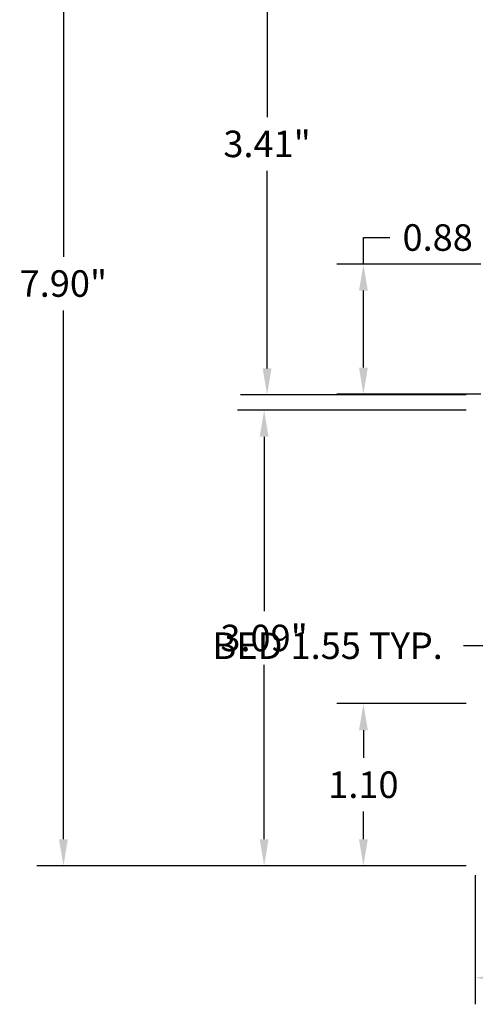
# Model space of a CAD drawing. Units: metres. Extents: x -1.9 to 13.1, y 0.9 to 14.8.
# Tile 1 of 7: x -1.9 to 1.2, y 1.8 to 8.4. Entities that reach past the tile are written whole.
import ezdxf

# ---------------------------------------------------------------- set-up
doc = ezdxf.new("R2010")
doc.units = ezdxf.units.M
doc.header["$MEASUREMENT"] = 0
doc.layers.add('A-ANNO-DIMS', color=2, linetype='Continuous', lineweight=13)
doc.styles.get("Standard").update_dxf_attribs({"font": 'arial.ttf'})
doc.dimstyles.get("Standard").update_dxf_attribs({"dimtxt": 0.18, "dimasz": 0.18, "dimexe": 0.18, "dimexo": 0.0625, "dimgap": 0.09, "dimtad": 0, "dimtih": 1, "dimtoh": 1, "dimzin": 0, "dimdsep": 46, "dimlunit": 3, "dimtxsty": 'Standard', "dimcen": 0.09, "dimadec": 0, "dimazin": 0, "dimtfac": 1, "dimtofl": 0, "dimtmove": 0, "dimatfit": 3, "dimfxl": 1, "dimtolj": 1, "dimtzin": 0, "dimarcsym": 0})

# ---------------------------------------------------------------- blocks, each defined once
blk = doc.blocks.new('*D20')
at = {"layer": 'A-ANNO-DIMS', "color": 0, "lineweight": -2, "transparency": 16777216}
for p, q in [((1.1413, 10.5964), (-1.7723, 10.5964)), ((-1.5923, 10.4164), (-1.5923, 6.8283)), ((-1.5923, 2.8764), (-1.5923, 6.4645)), ((1.1413, 2.6964), (-1.7723, 2.6964))]:
    blk.add_line(p, q, dxfattribs=at)
at = {"layer": 'A-ANNO-DIMS', "color": 0, "transparency": 16777216}
for points in [[(-1.6223, 10.4164), (-1.5623, 10.4164), (-1.5923, 10.5964)], [(-1.6223, 2.8764), (-1.5623, 2.8764), (-1.5923, 2.6964)]]:
    blk.add_solid(points, dxfattribs=at)
at = {"layer": 'Defpoints', "color": 0, "transparency": 16777216}
for p in [(1.2038, 10.5964), (-1.5923, 2.6964), (1.2038, 2.6964)]:
    blk.add_point(p, dxfattribs=at)
at = {"layer": 'A-ANNO-DIMS', "color": 0, "transparency": 16777216, "insert": (-1.5923, 6.6464), "char_height": 0.18, "attachment_point": 5}
blk.add_mtext('\\A1;7.90"', dxfattribs=at)
blk = doc.blocks.new('*D22')
at = {"layer": 'A-ANNO-DIMS', "color": 0, "lineweight": -2, "transparency": 16777216}
for p, q in [((1.1413, 9.2964), (-0.3896, 9.2964)), ((-0.2096, 9.1164), (-0.2096, 7.7756)), ((-0.2096, 6.0709), (-0.2096, 7.4117)), ((1.1413, 5.8909), (-0.3896, 5.8909))]:
    blk.add_line(p, q, dxfattribs=at)
at = {"layer": 'A-ANNO-DIMS', "color": 0, "transparency": 16777216}
for points in [[(-0.2396, 9.1164), (-0.1796, 9.1164), (-0.2096, 9.2964)], [(-0.2396, 6.0709), (-0.1796, 6.0709), (-0.2096, 5.8909)]]:
    blk.add_solid(points, dxfattribs=at)
at = {"layer": 'Defpoints', "color": 0, "transparency": 16777216}
for p in [(1.2038, 9.2964), (-0.2096, 5.8909), (1.2038, 5.8909)]:
    blk.add_point(p, dxfattribs=at)
at = {"layer": 'A-ANNO-DIMS', "color": 0, "transparency": 16777216, "insert": (-0.2096, 7.5936), "char_height": 0.18, "attachment_point": 5}
blk.add_mtext('\\A1;3.41"', dxfattribs=at)
blk = doc.blocks.new('*D23')
at = {"layer": 'A-ANNO-DIMS', "color": 0, "lineweight": -2, "transparency": 16777216}
for p, q in [((1.1413, 5.7874), (-0.4098, 5.7874)), ((-0.2298, 5.6074), (-0.2298, 4.4239)), ((-0.2298, 2.8764), (-0.2298, 4.0599)), ((1.1413, 2.6964), (-0.4098, 2.6964))]:
    blk.add_line(p, q, dxfattribs=at)
at = {"layer": 'A-ANNO-DIMS', "color": 0, "transparency": 16777216}
for points in [[(-0.2598, 5.6074), (-0.1998, 5.6074), (-0.2298, 5.7874)], [(-0.2598, 2.8764), (-0.1998, 2.8764), (-0.2298, 2.6964)]]:
    blk.add_solid(points, dxfattribs=at)
at = {"layer": 'Defpoints', "color": 0, "transparency": 16777216}
for p in [(1.2038, 5.7874), (-0.2298, 2.6964), (1.2038, 2.6964)]:
    blk.add_point(p, dxfattribs=at)
at = {"layer": 'A-ANNO-DIMS', "color": 0, "transparency": 16777216, "insert": (-0.2298, 4.2419), "char_height": 0.18, "attachment_point": 5}
blk.add_mtext('\\A1;3.09"', dxfattribs=at)
blk = doc.blocks.new('*D36')
at = {"layer": 'A-ANNO-DIMS', "color": 0, "lineweight": -2, "transparency": 16777216}
for p, q in [((1.3038, 4.0198), (1.3038, 4.3694)), ((2.8517, 4.0198), (2.8517, 4.3694)), ((1.3038, 4.1894), (1.1238, 4.1894)), ((2.6717, 4.1894), (1.4838, 4.1894))]:
    blk.add_line(p, q, dxfattribs=at)
at = {"layer": 'A-ANNO-DIMS', "color": 0, "transparency": 16777216}
for points in [[(1.4838, 4.2194), (1.4838, 4.1594), (1.3038, 4.1894)], [(2.6717, 4.2194), (2.6717, 4.1594), (2.8517, 4.1894)]]:
    blk.add_solid(points, dxfattribs=at)
at = {"layer": 'Defpoints', "color": 0, "transparency": 16777216}
for p in [(1.3038, 4.1894), (1.3038, 3.9573), (2.8517, 3.9573)]:
    blk.add_point(p, dxfattribs=at)
at = {"layer": 'A-ANNO-DIMS', "color": 0, "transparency": 16777216, "insert": (0.2014, 4.1894), "char_height": 0.18, "attachment_point": 5}
blk.add_mtext('\\A1;BED 1.55 TYP.', dxfattribs=at)
blk = doc.blocks.new('*D50')
at = {"layer": 'A-ANNO-DIMS', "color": 0, "lineweight": -2, "transparency": 16777216}
for p, q in [((1.203847, 2.633878), (1.203847, 1.756878)), ((2.403847, 2.633878), (2.403847, 1.756878)), ((1.383847, 1.936878), (1.488847, 1.936878)), ((2.223847, 1.936878), (2.118847, 1.936878))]:
    blk.add_line(p, q, dxfattribs=at)
at = {"layer": 'A-ANNO-DIMS', "color": 0, "transparency": 16777216}
for points in [[(1.383847, 1.966878), (1.383847, 1.906878), (1.203847, 1.936878)], [(2.223847, 1.966878), (2.223847, 1.906878), (2.403847, 1.936878)]]:
    blk.add_solid(points, dxfattribs=at)
at = {"layer": 'Defpoints', "color": 0, "transparency": 16777216}
for p in [(1.203847, 2.696378), (2.403847, 2.696378), (2.403847, 1.936878)]:
    blk.add_point(p, dxfattribs=at)
at = {"layer": 'A-ANNO-DIMS', "color": 0, "transparency": 16777216, "insert": (1.803847, 1.936878), "char_height": 0.18, "attachment_point": 5}
blk.add_mtext('\\A1;1.20', dxfattribs=at)
blk = doc.blocks.new('*D51')
at = {"layer": 'A-ANNO-DIMS', "color": 0, "lineweight": -2, "transparency": 16777216}
for p, q in [((1.1413, 3.7964), (0.2643, 3.7964)), ((0.4443, 3.6164), (0.4443, 3.4283)), ((0.4443, 2.8764), (0.4443, 3.0645)), ((1.1413, 2.6964), (0.2643, 2.6964))]:
    blk.add_line(p, q, dxfattribs=at)
at = {"layer": 'A-ANNO-DIMS', "color": 0, "transparency": 16777216}
for points in [[(0.4143, 3.6164), (0.4743, 3.6164), (0.4443, 3.7964)], [(0.4143, 2.8764), (0.4743, 2.8764), (0.4443, 2.6964)]]:
    blk.add_solid(points, dxfattribs=at)
at = {"layer": 'Defpoints', "color": 0, "transparency": 16777216}
for p in [(0.4443, 3.7964), (1.2038, 3.7964), (1.2038, 2.6964)]:
    blk.add_point(p, dxfattribs=at)
at = {"layer": 'A-ANNO-DIMS', "color": 0, "transparency": 16777216, "insert": (0.4443, 3.2464), "char_height": 0.18, "attachment_point": 5}
blk.add_mtext('\\A1;1.10', dxfattribs=at)
blk = doc.blocks.new('*D52')
at = {"layer": 'A-ANNO-DIMS', "color": 0, "lineweight": -2, "transparency": 16777216}
for p, q in [((0.4443, 6.7785), (0.4443, 6.9585)), ((0.4443, 6.9585), (0.6243, 6.9585)), ((1.2413, 6.7785), (0.2643, 6.7785)), ((0.4443, 6.0764), (0.4443, 6.5985)), ((1.2413, 5.8964), (0.2643, 5.8964))]:
    blk.add_line(p, q, dxfattribs=at)
at = {"layer": 'A-ANNO-DIMS', "color": 0, "transparency": 16777216}
for points in [[(0.4143, 6.5985), (0.4743, 6.5985), (0.4443, 6.7785)], [(0.4143, 6.0764), (0.4743, 6.0764), (0.4443, 5.8964)]]:
    blk.add_solid(points, dxfattribs=at)
at = {"layer": 'Defpoints', "color": 0, "transparency": 16777216}
for p in [(0.4443, 6.7785), (1.3038, 6.7785), (1.3038, 5.8964)]:
    blk.add_point(p, dxfattribs=at)
at = {"layer": 'A-ANNO-DIMS', "color": 0, "transparency": 16777216, "insert": (0.9483, 6.9585), "char_height": 0.18, "attachment_point": 5}
blk.add_mtext('\\A1;0.88', dxfattribs=at)

msp = doc.modelspace()

# ---------------------------------------------------------------- dimensions: what is measured, and where the dimension line sits
at = {"layer": 'A-ANNO-DIMS'}
for base, p1, p2, override, picture, middle in [((-1.5923, 2.6964), (1.2038, 10.5964), (1.2038, 2.6964), {"dimclrd": 0, "dimclre": 0, "dimclrt": 0}, '*D20', (-1.5923, 6.6464)), ((-0.2096, 5.8909), (1.2038, 9.2964), (1.2038, 5.8909), {"dimclrd": 0, "dimclre": 0, "dimclrt": 0}, '*D22', (-0.2096, 7.5936)), ((0.4443, 6.7785), (1.3038, 5.8964), (1.3038, 6.7785), {"dimdec": 2, "dimlfac": 1, "dimrnd": 0, "dimzin": 0, "dimdsep": 46, "dimlunit": 2}, '*D52', (0.9483, 6.9585)), ((-0.2298, 2.6964), (1.2038, 5.7874), (1.2038, 2.6964), {"dimclrd": 0, "dimclre": 0, "dimclrt": 0}, '*D23', (-0.2298, 4.2419)), ((0.4443, 3.7964), (1.2038, 2.6964), (1.2038, 3.7964), {"dimdec": 2, "dimlfac": 1, "dimrnd": 0, "dimzin": 0, "dimdsep": 46, "dimlunit": 2}, '*D51', (0.4443, 3.2464))]:
    dim = msp.add_linear_dim(base=base, p1=p1, p2=p2, angle=90, dimstyle='Standard', override=override, dxfattribs=at)
    dim.commit()
    dim.dimension.update_dxf_attribs({"geometry": picture, "text_midpoint": middle})
dim = msp.add_linear_dim(base=(1.3038, 4.1894), p1=(2.8517, 3.9573), p2=(1.3038, 3.9573), angle=180, text='BED <> TYP.', dimstyle='Standard', override={"dimdec": 2, "dimlfac": 1, "dimrnd": 0, "dimzin": 0, "dimdsep": 46, "dimlunit": 2}, dxfattribs=at)
dim.commit()
dim.dimension.update_dxf_attribs({"geometry": '*D36', "text_midpoint": (0.2014, 4.1894)})
dim = msp.add_linear_dim(base=(2.4038, 1.9369), p1=(1.2038, 2.6964), p2=(2.4038, 2.6964), dimstyle='Standard', override={"dimdec": 2, "dimlfac": 1, "dimrnd": 0, "dimzin": 0, "dimdsep": 46, "dimlunit": 2}, dxfattribs=at)
dim.commit()
dim.dimension.update_dxf_attribs({"geometry": '*D50', "text_midpoint": (1.8038, 1.9369)})

doc.saveas('drawing.dxf')
